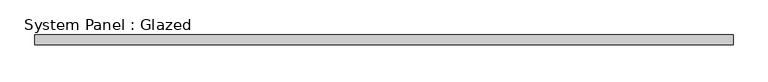
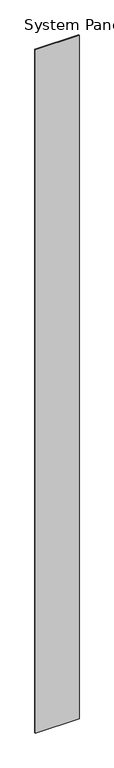
"""IFC4 building model written with IfcOpenShell, lengths in millimetres: plate geometry, System Panel : Glazed."""

from ifc_helpers import new_model, si_unit, origin, origin_with_axes, place, context, project, spatial, polyline, outline, extrude, source, transform, mapped, element, save


def system_panel_glazed_c868bc05(model_context):
    return source(origin(), model_context, "Body", "SweptSolid", [
        extrude(outline(polyline([(882.65, 19.05), (-882.65, 19.05), (-882.65, 44.45), (882.65, 44.45), (882.65, 19.05)])), origin_with_axes(), (0.0, 0.0, 1.0), 29133.8),
    ])


if __name__ == "__main__":
    model = new_model("IFC4")
    model_context = context("Model", 3, world=origin())
    ifc_project = project(units=[si_unit("LENGTHUNIT", "METRE", prefix="MILLI")], contexts=[model_context])
    site = spatial("IfcSite", under=ifc_project)
    building = spatial("IfcBuilding", under=site)
    placement = place(None, origin())
    system_panel_glazed_shape = system_panel_glazed_c868bc05(model_context)
    element("IfcPlate", 1, ObjectType="System Panel : Glazed", at=placement, inside=building, context=model_context, shape_type="MappedRepresentation", body=[
        mapped(system_panel_glazed_shape, transform((0.0, 0.0, 0.0), x_axis=(1.0, 0.0, 0.0), y_axis=(0.0, 1.0, 0.0), z_axis=(0.0, 0.0, 1.0))),
    ])
    save(model, "model.ifc")

# Revit data of these elements
# Type "System Panel : Glazed"
#   Construction Type Id = "GSP4R"
#   Analytic Construction = "1/8 in Pilkington single glazing"
#   Visual Light Transmittance = 0.9
#   Solar Heat Gain Coefficient = 0.86
#   Heat Transfer Coefficient (U) = 1.18115 BTU/(h·ft²·°F)
# Element 1 (IfcPlate, "System Panel : Glazed")
#   Materials on its faces: "Glass"
# Materials
#   "Glass": class "Glass", colour RGB 0 128 192, transparency 0.75, Description = "Soda Lime Glass", Cost = 0
